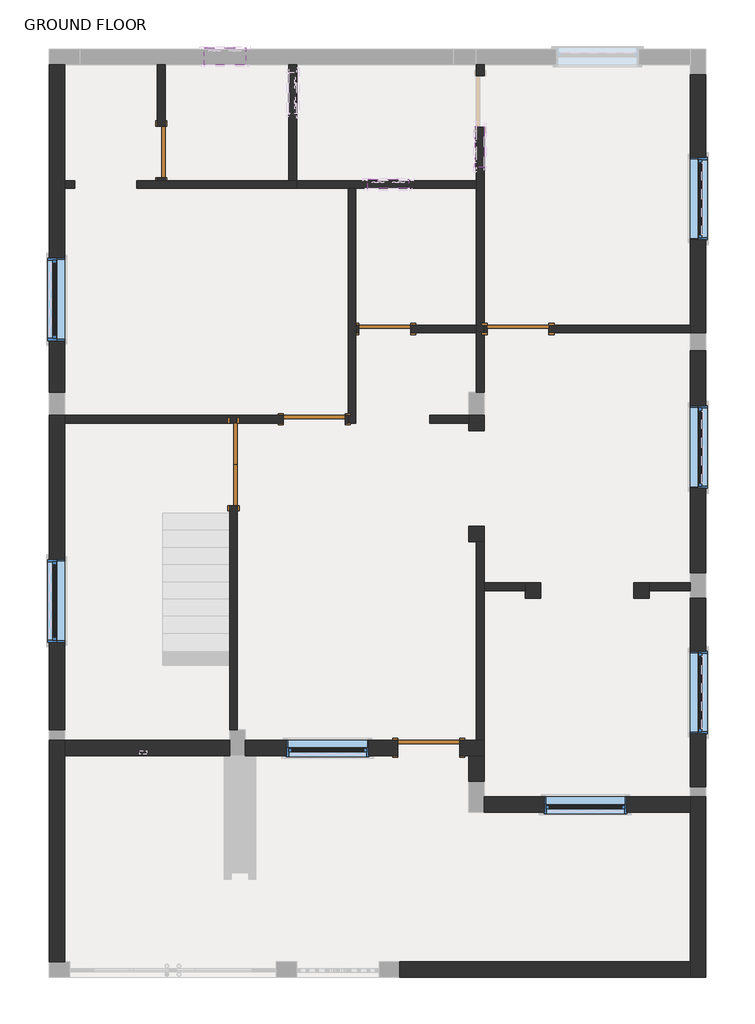
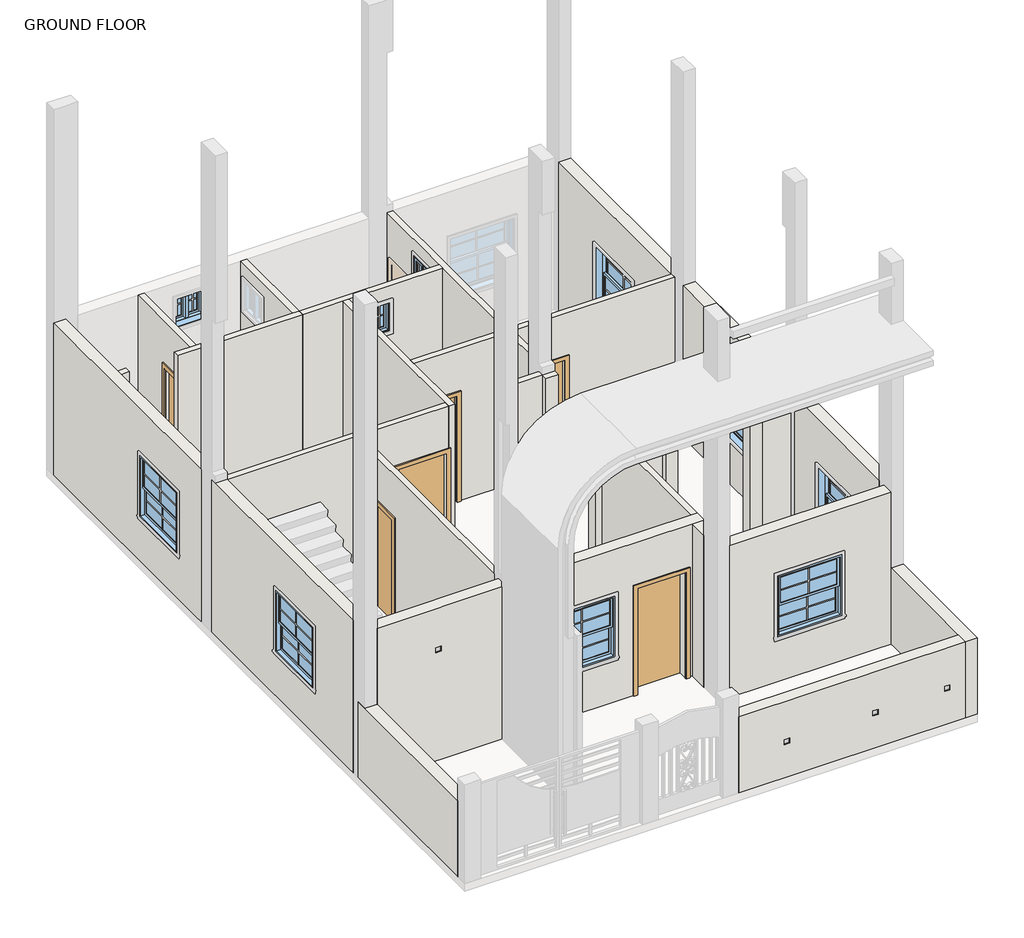
# One storey, part 1 of 3: 31 walls, 10 windows, 6 doors.
"""IFC4 building model written with IfcOpenShell, lengths in millimetres."""

from ifc_helpers import new_model, si_unit, frame, origin, origin_with_axes, place, context, project, spatial, polyline, outline, extrude, faceted_brep, transform, mapped, element, save
from components import door_double_flush_panel_4_x7_eb8a45e1, door_78caadf7, door_214872d5, single_flush_3_x7_0ca8825f, single_flush_3_x7_e5f9f3c4, single_flush_3_x7_305aa2a5, window_casement_double_2_x2_e4709907, window_casement_double_2_x2_3fc3773f, window_double_hung_4_x4_ec8efb0e

model = new_model("IFC4")

# Units and contexts
model_context = context("Model", 3, world=origin())
ifc_project = project(units=[si_unit("LENGTHUNIT", "METRE", prefix="MILLI")], contexts=[model_context])

# Site, building, storey
site = spatial("IfcSite", under=ifc_project)
building = spatial("IfcBuilding", under=site)
storey = spatial("IfcBuildingStorey", under=building, Name="GROUND FLOOR", Elevation=0.0)

# Doors
placement = place(None, origin())
door_double_flush_panel_4_x7_shape = door_double_flush_panel_4_x7_eb8a45e1(model_context)
element("IfcDoor", 1, ObjectType="Door-Double-Flush_Panel : 4'X7'", at=placement, inside=storey, context=model_context, shape_type="MappedRepresentation", body=[
    mapped(door_double_flush_panel_4_x7_shape, transform((-10167.2709734, 2753.6170657, 0.0), x_axis=(0.0, -1.0, 0.0), y_axis=(1.0, 0.0, 0.0), z_axis=(0.0, 0.0, 1.0))),
])
door_shape = door_78caadf7(model_context)
element("IfcDoor", 2, ObjectType="Single-Flush : 2'6\"", at=placement, inside=storey, context=model_context, shape_type="MappedRepresentation", body=[
    mapped(door_shape, transform((-7932.0709734, 4753.8670657, 0.0), x_axis=(-1.0, 0.0, 0.0), y_axis=(0.0, -1.0, 0.0), z_axis=(0.0, 0.0, 1.0))),
])
door_2_shape = door_214872d5(model_context)
element("IfcDoor", 3, ObjectType="Single-Flush : 2'6\"", at=placement, inside=storey, context=model_context, shape_type="MappedRepresentation", body=[
    mapped(door_2_shape, transform((-11234.0709734, 7370.0670657, 0.0), x_axis=(0.0, -1.0, 0.0), y_axis=(1.0, 0.0, 0.0), z_axis=(0.0, 0.0, 1.0))),
])
single_flush_3_x7_shape = single_flush_3_x7_0ca8825f(model_context)
element("IfcDoor", 4, ObjectType="Single-Flush : 3'X7'", at=placement, inside=storey, context=model_context, shape_type="MappedRepresentation", body=[
    mapped(single_flush_3_x7_shape, transform((-7284.3709734, -1437.3829343, 0.0), x_axis=(1.0, 0.0, 0.0), y_axis=(0.0, 1.0, 0.0), z_axis=(0.0, 0.0, 1.0))),
])
single_flush_3_x7_2_shape = single_flush_3_x7_e5f9f3c4(model_context)
element("IfcDoor", 5, ObjectType="Single-Flush : 3'X7'", at=placement, inside=storey, context=model_context, shape_type="MappedRepresentation", body=[
    mapped(single_flush_3_x7_2_shape, transform((-8973.4709734, 3420.3670657, 0.0), x_axis=(1.0, 0.0, 0.0), y_axis=(0.0, 1.0, 0.0), z_axis=(0.0, 0.0, 1.0))),
])
single_flush_3_x7_3_shape = single_flush_3_x7_305aa2a5(model_context)
element("IfcDoor", 6, ObjectType="Single-Flush : 3'X7'", at=placement, inside=storey, context=model_context, shape_type="MappedRepresentation", body=[
    mapped(single_flush_3_x7_3_shape, transform((-5963.5709734, 4753.8670657, 0.0), x_axis=(-1.0, 0.0, 0.0), y_axis=(0.0, -1.0, 0.0), z_axis=(0.0, 0.0, 1.0))),
])

# Walls
element("IfcWall", 7, ObjectType="4.5\"", at=placement, inside=storey, context=model_context, shape_type="SweptSolid", body=[
    extrude(outline(polyline([(-12510.4209734, 6830.3170657), (-12662.8209734, 6830.3170657), (-12662.8209734, 6944.6170657), (-12510.4209734, 6944.6170657), (-12510.4209734, 6830.3170657)])), origin_with_axes(), (0.0, 0.0, 1.0), 3048.0),
])
element("IfcWall", 8, ObjectType="4.5\"", at=placement, inside=storey, context=model_context, shape_type="Brep", body=[
    faceted_brep([(-11596.0209734, 6830.3170657, 0.0), (-9233.8209734, 6830.3170657, 0.0), (-9233.8209734, 6830.3170657, 3048.0), (-11596.0209734, 6830.3170657, 3048.0), (-11596.0209734, 6944.6170657, 0.0), (-11596.0209734, 6944.6170657, 3048.0), (-11291.2209734, 6944.6170657, 3048.0), (-11176.9209734, 6944.6170657, 3048.0), (-9348.1209734, 6944.6170657, 3048.0), (-9233.8209734, 6944.6170657, 3048.0), (-9233.8209734, 6944.6170657, 0.0), (-9348.1209734, 6944.6170657, 0.0), (-11176.9209734, 6944.6170657, 0.0), (-11291.2209734, 6944.6170657, 0.0)], [[[0, 1, 2, 3]], [[4, 5, 6, 7, 8, 9, 10, 11, 12, 13]], [[1, 0, 4, 13, 12, 11, 10]], [[3, 2, 9, 8, 7, 6, 5]], [[0, 3, 5, 4]], [[2, 1, 10, 9]]]),
])
element("IfcWall", 9, ObjectType="4.5\"", at=placement, inside=storey, context=model_context, shape_type="SweptSolid", body=[
    extrude(outline(polyline([(6944.6170657, 0.0), (6944.6170657, 3048.0), (8659.1170657, 3048.0), (8659.1170657, 0.0), (6944.6170657, 0.0)]), holes=[polyline([(7935.2170657, 2743.2), (7935.2170657, 2133.6), (8544.8170657, 2133.6), (8544.8170657, 2743.2), (7935.2170657, 2743.2)])]), frame((-9348.1209734, 0.0, 0.0), z_axis=(1.0, 0.0, 0.0), x_axis=(0.0, 1.0, 0.0)), (0.0, 0.0, 1.0), 114.3),
])
element("IfcWall", 10, ObjectType="4.5\"", at=placement, inside=storey, context=model_context, shape_type="SweptSolid", body=[
    extrude(outline(polyline([(6989.0670657, 2133.6), (6989.0670657, 0.0), (6944.6170657, 0.0), (6944.6170657, 3048.0), (8659.1170657, 3048.0), (8659.1170657, 0.0), (7751.0670657, 0.0), (7751.0670657, 2133.6), (6989.0670657, 2133.6)])), frame((-11291.2209734, 0.0, 0.0), z_axis=(1.0, 0.0, 0.0), x_axis=(0.0, 1.0, 0.0)), (0.0, 0.0, 1.0), 114.3),
])
element("IfcWall", 11, ObjectType="4.5\"", at=placement, inside=storey, context=model_context, shape_type="Brep", body=[
    faceted_brep([(-6579.5209734, 6944.6170657, 0.0), (-9233.8209734, 6944.6170657, 0.0), (-9233.8209734, 6944.6170657, 3048.0), (-6579.5209734, 6944.6170657, 3048.0), (-7576.4709734, 6944.6170657, 2743.2), (-8186.0709734, 6944.6170657, 2743.2), (-8186.0709734, 6944.6170657, 2133.6), (-7576.4709734, 6944.6170657, 2133.6), (-6579.5209734, 6830.3170657, 0.0), (-6579.5209734, 6830.3170657, 3048.0), (-8357.5209734, 6830.3170657, 3048.0), (-8471.8209734, 6830.3170657, 3048.0), (-9233.8209734, 6830.3170657, 3048.0), (-9233.8209734, 6830.3170657, 0.0), (-8471.8209734, 6830.3170657, 0.0), (-8357.5209734, 6830.3170657, 0.0), (-7576.4709734, 6830.3170657, 2743.2), (-7576.4709734, 6830.3170657, 2133.6), (-8186.0709734, 6830.3170657, 2133.6), (-8186.0709734, 6830.3170657, 2743.2)], [[[0, 1, 2, 3], [4, 5, 6, 7]], [[8, 9, 10, 11, 12, 13, 14, 15], [16, 17, 18, 19]], [[1, 0, 8, 15, 14, 13]], [[3, 2, 12, 11, 10, 9]], [[2, 1, 13, 12]], [[0, 3, 9, 8]], [[17, 16, 4, 7]], [[18, 17, 7, 6]], [[19, 18, 6, 5]], [[16, 19, 5, 4]]]),
])
element("IfcWall", 12, ObjectType="4.5\"", at=placement, inside=storey, context=model_context, shape_type="Brep", body=[
    faceted_brep([(-6579.5209734, 3820.4170657, 0.0), (-6579.5209734, 3820.4170657, 3048.0), (-6579.5209734, 4696.7170657, 3048.0), (-6579.5209734, 4811.0170657, 3048.0), (-6579.5209734, 6830.3170657, 3048.0), (-6579.5209734, 6944.6170657, 3048.0), (-6579.5209734, 8659.1170657, 3048.0), (-6579.5209734, 8659.1170657, 0.0), (-6579.5209734, 8494.0170657, 0.0), (-6579.5209734, 8494.0170657, 2133.6), (-6579.5209734, 7751.0670657, 2133.6), (-6579.5209734, 7751.0670657, 2743.2), (-6579.5209734, 7141.4670657, 2743.2), (-6579.5209734, 7141.4670657, 2133.6), (-6579.5209734, 7732.0170657, 2133.6), (-6579.5209734, 7732.0170657, 0.0), (-6579.5209734, 6944.6170657, 0.0), (-6579.5209734, 6830.3170657, 0.0), (-6579.5209734, 4811.0170657, 0.0), (-6579.5209734, 4696.7170657, 0.0), (-6465.2209734, 3820.4170657, 3048.0), (-6465.2209734, 3820.4170657, 0.0), (-6465.2209734, 4696.7170657, 0.0), (-6465.2209734, 4811.0170657, 0.0), (-6465.2209734, 7732.0170657, 0.0), (-6465.2209734, 7732.0170657, 2133.6), (-6465.2209734, 7141.4670657, 2133.6), (-6465.2209734, 7141.4670657, 2743.2), (-6465.2209734, 7751.0670657, 2743.2), (-6465.2209734, 7751.0670657, 2133.6), (-6465.2209734, 8494.0170657, 2133.6), (-6465.2209734, 8494.0170657, 0.0), (-6465.2209734, 8659.1170657, 0.0), (-6465.2209734, 8659.1170657, 3048.0), (-6465.2209734, 4811.0170657, 3048.0), (-6465.2209734, 4696.7170657, 3048.0)], [[[0, 1, 2, 3, 4, 5, 6, 7, 8, 9, 10, 11, 12, 13, 14, 15, 16, 17, 18, 19]], [[20, 21, 22, 23, 24, 25, 26, 27, 28, 29, 30, 31, 32, 33, 34, 35]], [[7, 32, 31, 8]], [[21, 0, 19, 18, 17, 16, 15, 24, 23, 22]], [[1, 0, 21, 20]], [[6, 5, 4, 3, 2, 1, 20, 35, 34, 33]], [[7, 6, 33, 32]], [[9, 8, 31, 30]], [[9, 30, 29, 10]], [[15, 14, 25, 24]], [[28, 11, 10, 29]], [[13, 26, 25, 14]], [[26, 13, 12, 27]], [[11, 28, 27, 12]]]),
])
element("IfcWall", 13, ObjectType="4.5\"", at=placement, inside=storey, context=model_context, shape_type="Brep", body=[
    faceted_brep([(-8471.8209734, 6830.3170657, 0.0), (-8471.8209734, 3477.5170657, 0.0), (-8471.8209734, 3363.2170657, 0.0), (-8471.8209734, 3363.2170657, 3048.0), (-8471.8209734, 3477.5170657, 3048.0), (-8471.8209734, 6830.3170657, 3048.0), (-8357.5209734, 6830.3170657, 0.0), (-8357.5209734, 6830.3170657, 3048.0), (-8357.5209734, 4811.0170657, 3048.0), (-8357.5209734, 4696.7170657, 3048.0), (-8357.5209734, 3363.2170657, 3048.0), (-8357.5209734, 3363.2170657, 0.0), (-8357.5209734, 4696.7170657, 0.0), (-8357.5209734, 4811.0170657, 0.0)], [[[0, 1, 2, 3, 4, 5]], [[6, 7, 8, 9, 10, 11, 12, 13]], [[2, 1, 0, 6, 13, 12, 11]], [[5, 4, 3, 10, 9, 8, 7]], [[0, 5, 7, 6]], [[3, 2, 11, 10]]]),
])
element("IfcWall", 14, ObjectType="4.5\"", at=placement, inside=storey, context=model_context, shape_type="SweptSolid", body=[
    extrude(outline(polyline([(-7265.3209734, 3477.5170657), (-6693.8209734, 3477.5170657), (-6693.8209734, 3363.2170657), (-7265.3209734, 3363.2170657), (-7265.3209734, 3477.5170657)])), origin_with_axes(), (0.0, 0.0, 1.0), 3048.0),
])
element("IfcWall", 15, ObjectType="4.5\"", at=placement, inside=storey, context=model_context, shape_type="SweptSolid", body=[
    extrude(outline(polyline([(0.0, -8357.5209734), (0.0, -8313.0709734), (2133.6, -8313.0709734), (2133.6, -7551.0709734), (0.0, -7551.0709734), (0.0, -6579.5209734), (3048.0, -6579.5209734), (3048.0, -8357.5209734), (0.0, -8357.5209734)])), frame((0.0, 4696.7170657, 0.0), z_axis=(0.0, 1.0, 0.0), x_axis=(0.0, 0.0, 1.0)), (0.0, 0.0, 1.0), 114.3),
])
element("IfcWall", 16, ObjectType="4.5\"", at=placement, inside=storey, context=model_context, shape_type="SweptSolid", body=[
    extrude(outline(polyline([(0.0, -6465.2209734), (0.0, -6420.7709734), (2133.6, -6420.7709734), (2133.6, -5506.3709734), (0.0, -5506.3709734), (0.0, -3417.2209734), (3048.0, -3417.2209734), (3048.0, -6465.2209734), (0.0, -6465.2209734)])), frame((0.0, 4696.7170657, 0.0), z_axis=(0.0, 1.0, 0.0), x_axis=(0.0, 0.0, 1.0)), (0.0, 0.0, 1.0), 114.3),
])
element("IfcWall", 17, ObjectType="4.5\"", at=placement, inside=storey, context=model_context, shape_type="Brep", body=[
    faceted_brep([(-8471.8209734, 3477.5170657, 0.0), (-8516.2709734, 3477.5170657, 0.0), (-8516.2709734, 3477.5170657, 2133.6), (-9430.6709734, 3477.5170657, 2133.6), (-9430.6709734, 3477.5170657, 0.0), (-12662.8209734, 3477.5170657, 0.0), (-12662.8209734, 3477.5170657, 3048.0), (-8471.8209734, 3477.5170657, 3048.0), (-8516.2709734, 3363.2170657, 2133.6), (-8516.2709734, 3363.2170657, 0.0), (-8471.8209734, 3363.2170657, 0.0), (-8471.8209734, 3363.2170657, 3048.0), (-10110.1209734, 3363.2170657, 3048.0), (-10224.4209734, 3363.2170657, 3048.0), (-12662.8209734, 3363.2170657, 3048.0), (-12662.8209734, 3363.2170657, 0.0), (-9430.6709734, 3363.2170657, 0.0), (-9430.6709734, 3363.2170657, 2133.6)], [[[0, 1, 2, 3, 4, 5, 6, 7]], [[8, 9, 10, 11, 12, 13, 14, 15, 16, 17]], [[16, 15, 5, 4]], [[10, 9, 1, 0]], [[7, 6, 14, 13, 12, 11]], [[6, 5, 15, 14]], [[0, 7, 11, 10]], [[2, 1, 9, 8]], [[3, 2, 8, 17]], [[4, 3, 17, 16]]]),
])
element("IfcWall", 18, ObjectType="4.5\"", at=placement, inside=storey, context=model_context, shape_type="SweptSolid", body=[
    extrude(outline(polyline([(-1170.6829343, 3048.0), (3363.2170657, 3048.0), (3363.2170657, 2133.6), (2144.0170657, 2133.6), (2144.0170657, 0.0), (-1170.6829343, 0.0), (-1170.6829343, 3048.0)])), frame((-10224.4209734, 0.0, 0.0), z_axis=(1.0, 0.0, 0.0), x_axis=(0.0, 1.0, 0.0)), (0.0, 0.0, 1.0), 114.3),
])
element("IfcWall", 19, ObjectType="4.5\"", at=placement, inside=storey, context=model_context, shape_type="SweptSolid", body=[
    extrude(outline(polyline([(-4026.8209734, 1001.0170657), (-3417.2209734, 1001.0170657), (-3417.2209734, 886.7170657), (-4026.8209734, 886.7170657), (-4026.8209734, 1001.0170657)])), origin_with_axes(), (0.0, 0.0, 1.0), 3048.0),
])
element("IfcWall", 20, ObjectType="4.5\"", at=placement, inside=storey, context=model_context, shape_type="Brep", body=[
    faceted_brep([(-6579.5209734, 1610.6170657, 0.0), (-6579.5209734, -1323.0829343, 0.0), (-6579.5209734, -1323.0829343, 3048.0), (-6579.5209734, 1610.6170657, 3048.0), (-6465.2209734, 1610.6170657, 0.0), (-6465.2209734, 1610.6170657, 3048.0), (-6465.2209734, 1001.0170657, 3048.0), (-6465.2209734, 886.7170657, 3048.0), (-6465.2209734, -1323.0829343, 3048.0), (-6465.2209734, -1323.0829343, 0.0), (-6465.2209734, 886.7170657, 0.0), (-6465.2209734, 1001.0170657, 0.0)], [[[0, 1, 2, 3]], [[4, 5, 6, 7, 8, 9, 10, 11]], [[1, 0, 4, 11, 10, 9]], [[3, 2, 8, 7, 6, 5]], [[0, 3, 5, 4]], [[2, 1, 9, 8]]]),
])
element("IfcWall", 21, ObjectType="4.5\"", at=placement, inside=storey, context=model_context, shape_type="SweptSolid", body=[
    extrude(outline(polyline([(-5855.6209734, 886.7170657), (-6465.2209734, 886.7170657), (-6465.2209734, 1001.0170657), (-5855.6209734, 1001.0170657), (-5855.6209734, 886.7170657)])), origin_with_axes(), (0.0, 0.0, 1.0), 3048.0),
])
element("IfcWall", 22, ObjectType="9\"", at=placement, inside=storey, context=model_context, shape_type="Brep", body=[
    faceted_brep([(-12891.4209734, 8659.1170657, 0.0), (-12891.4209734, 3820.4170657, 0.0), (-12891.4209734, 3820.4170657, 3048.0), (-12891.4209734, 8659.1170657, 3048.0), (-12891.4209734, 4582.4170657, 2133.6), (-12891.4209734, 4582.4170657, 914.4), (-12891.4209734, 5801.6170657, 914.4), (-12891.4209734, 5801.6170657, 2133.6), (-12662.8209734, 8659.1170657, 0.0), (-12662.8209734, 8659.1170657, 3048.0), (-12662.8209734, 6944.6170657, 3048.0), (-12662.8209734, 6830.3170657, 3048.0), (-12662.8209734, 3820.4170657, 3048.0), (-12662.8209734, 3820.4170657, 0.0), (-12662.8209734, 6830.3170657, 0.0), (-12662.8209734, 6944.6170657, 0.0), (-12662.8209734, 4582.4170657, 2133.6), (-12662.8209734, 5801.6170657, 2133.6), (-12662.8209734, 5801.6170657, 914.4), (-12662.8209734, 4582.4170657, 914.4)], [[[0, 1, 2, 3], [4, 5, 6, 7]], [[8, 9, 10, 11, 12, 13, 14, 15], [16, 17, 18, 19]], [[1, 0, 8, 15, 14, 13]], [[2, 1, 13, 12]], [[3, 2, 12, 11, 10, 9]], [[0, 3, 9, 8]], [[5, 4, 16, 19]], [[6, 5, 19, 18]], [[7, 6, 18, 17]], [[4, 7, 17, 16]]]),
])
element("IfcWall", 23, ObjectType="9\"", at=placement, inside=storey, context=model_context, shape_type="Brep", body=[
    faceted_brep([(-12891.4209734, 3477.5170657, 0.0), (-12891.4209734, -1170.6829343, 0.0), (-12891.4209734, -1170.6829343, 3048.0), (-12891.4209734, 3363.2170657, 3048.0), (-12891.4209734, 3477.5170657, 3048.0), (-12891.4209734, 124.7170657, 2133.6), (-12891.4209734, 124.7170657, 914.4), (-12891.4209734, 1343.9170657, 914.4), (-12891.4209734, 1343.9170657, 2133.6), (-12662.8209734, 3477.5170657, 0.0), (-12662.8209734, 3477.5170657, 3048.0), (-12662.8209734, 3363.2170657, 3048.0), (-12662.8209734, -1170.6829343, 3048.0), (-12662.8209734, -1170.6829343, 0.0), (-12662.8209734, 3363.2170657, 0.0), (-12662.8209734, 124.7170657, 2133.6), (-12662.8209734, 1343.9170657, 2133.6), (-12662.8209734, 1343.9170657, 914.4), (-12662.8209734, 124.7170657, 914.4)], [[[0, 1, 2, 3, 4], [5, 6, 7, 8]], [[9, 10, 11, 12, 13, 14], [15, 16, 17, 18]], [[1, 0, 9, 14, 13]], [[2, 1, 13, 12]], [[4, 3, 2, 12, 11, 10]], [[0, 4, 10, 9]], [[6, 5, 15, 18]], [[7, 6, 18, 17]], [[8, 7, 17, 16]], [[5, 8, 16, 15]]]),
])
element("IfcWall", 24, ObjectType="9\"", at=placement, inside=storey, context=model_context, shape_type="Brep", body=[
    faceted_brep([(-12891.4209734, -1323.0829343, 0.0), (-12891.4209734, -4599.6829343, 0.0), (-12891.4209734, -4599.6829343, 1524.0), (-12891.4209734, -1551.6829343, 1524.0), (-12891.4209734, -1323.0829343, 1524.0), (-12662.8209734, -1323.0829343, 0.0), (-12662.8209734, -1323.0829343, 1524.0), (-12662.8209734, -1551.6829343, 1524.0), (-12662.8209734, -4599.6829343, 1524.0), (-12662.8209734, -4599.6829343, 0.0), (-12662.8209734, -1551.6829343, 0.0)], [[[0, 1, 2, 3, 4]], [[5, 6, 7, 8, 9, 10]], [[1, 0, 5, 10, 9]], [[2, 1, 9, 8]], [[4, 3, 2, 8, 7, 6]], [[0, 4, 6, 5]]]),
])
element("IfcWall", 25, ObjectType="9\"", at=placement, inside=storey, context=model_context, shape_type="Brep", body=[
    faceted_brep([(-3417.2209734, 8506.7170657, 0.0), (-3417.2209734, 4811.0170657, 0.0), (-3417.2209734, 4696.7170657, 0.0), (-3417.2209734, 4696.7170657, 3048.0), (-3417.2209734, 4811.0170657, 3048.0), (-3417.2209734, 8506.7170657, 3048.0), (-3417.2209734, 7287.5170657, 2133.6), (-3417.2209734, 6068.3170657, 2133.6), (-3417.2209734, 6068.3170657, 914.4), (-3417.2209734, 7287.5170657, 914.4), (-3188.6209734, 8506.7170657, 0.0), (-3188.6209734, 8506.7170657, 3048.0), (-3188.6209734, 4811.0170657, 3048.0), (-3188.6209734, 4696.7170657, 3048.0), (-3188.6209734, 4696.7170657, 0.0), (-3188.6209734, 7287.5170657, 2133.6), (-3188.6209734, 7287.5170657, 914.4), (-3188.6209734, 6068.3170657, 914.4), (-3188.6209734, 6068.3170657, 2133.6)], [[[0, 1, 2, 3, 4, 5], [6, 7, 8, 9]], [[10, 11, 12, 13, 14], [15, 16, 17, 18]], [[2, 1, 0, 10, 14]], [[5, 4, 3, 13, 12, 11]], [[0, 5, 11, 10]], [[3, 2, 14, 13]], [[16, 15, 6, 9]], [[17, 16, 9, 8]], [[18, 17, 8, 7]], [[15, 18, 7, 6]]]),
])
element("IfcWall", 26, ObjectType="9\"", at=placement, inside=storey, context=model_context, shape_type="SweptSolid", body=[
    extrude(outline(polyline([(4430.0170657, 0.0), (1153.4170657, 0.0), (1153.4170657, 3048.0), (4430.0170657, 3048.0), (4430.0170657, 0.0)]), holes=[polyline([(3617.2170657, 2133.6), (2398.0170657, 2133.6), (2398.0170657, 914.4), (3617.2170657, 914.4), (3617.2170657, 2133.6)])]), frame((-3417.2209734, 0.0, 0.0), z_axis=(1.0, 0.0, 0.0), x_axis=(0.0, 1.0, 0.0)), (0.0, 0.0, 1.0), 228.6),
])
element("IfcWall", 27, ObjectType="9\"", at=placement, inside=storey, context=model_context, shape_type="SweptSolid", body=[
    extrude(outline(polyline([(772.4170657, 0.0), (-2008.8829343, 0.0), (-2008.8829343, 3048.0), (772.4170657, 3048.0), (772.4170657, 0.0)]), holes=[polyline([(-8.6329343, 2133.6), (-1227.8329343, 2133.6), (-1227.8329343, 914.4), (-8.6329343, 914.4), (-8.6329343, 2133.6)])]), frame((-3417.2209734, 0.0, 0.0), z_axis=(1.0, 0.0, 0.0), x_axis=(0.0, 1.0, 0.0)), (0.0, 0.0, 1.0), 228.6),
])
element("IfcWall", 28, ObjectType="9\"", at=placement, inside=storey, context=model_context, shape_type="Brep", body=[
    faceted_brep([(-3417.2209734, -2161.2829343, 0.0), (-3417.2209734, -2389.8829343, 0.0), (-3417.2209734, -4599.6829343, 0.0), (-3417.2209734, -4828.2829343, 0.0), (-3417.2209734, -4828.2829343, 1524.0), (-3417.2209734, -4599.6829343, 1524.0), (-3417.2209734, -2389.8829343, 1524.0), (-3417.2209734, -2161.2829343, 1524.0), (-3188.6209734, -2161.2829343, 0.0), (-3188.6209734, -2161.2829343, 1524.0), (-3188.6209734, -2389.8829343, 1524.0), (-3188.6209734, -4828.2829343, 1524.0), (-3188.6209734, -4828.2829343, 0.0)], [[[0, 1, 2, 3, 4, 5, 6, 7]], [[8, 9, 10, 11, 12]], [[3, 2, 1, 0, 8, 12]], [[7, 6, 5, 4, 11, 10, 9]], [[4, 3, 12, 11]], [[0, 7, 9, 8]]]),
])
element("IfcWall", 29, ObjectType="9\"", at=placement, inside=storey, context=model_context, shape_type="SweptSolid", body=[
    extrude(outline(polyline([(0.0, -3417.2209734), (1524.0, -3417.2209734), (1524.0, -7709.8209734), (0.0, -7709.8209734), (0.0, -3417.2209734)]), holes=[polyline([(763.994346, -6745.4209734), (663.994346, -6745.4209734), (663.994346, -6845.4209734), (763.994346, -6845.4209734), (763.994346, -6745.4209734)]), polyline([(751.9195264, -5069.0209734), (651.9195264, -5069.0209734), (651.9195264, -5169.0209734), (751.9195264, -5169.0209734), (751.9195264, -5069.0209734)]), polyline([(769.6864335, -3710.1209734), (669.6864335, -3710.1209734), (669.6864335, -3810.1209734), (769.6864335, -3810.1209734), (769.6864335, -3710.1209734)])]), frame((0.0, -4828.2829343, 0.0), z_axis=(0.0, 1.0, 0.0), x_axis=(0.0, 0.0, 1.0)), (0.0, 0.0, 1.0), 228.6),
])
element("IfcWall", 30, ObjectType="9\"", at=placement, inside=storey, context=model_context, shape_type="Brep", body=[
    faceted_brep([(-6827.1709734, -1551.6829343, 2133.6), (-6827.1709734, -1551.6829343, 0.0), (-6693.8209734, -1551.6829343, 0.0), (-6465.2209734, -1551.6829343, 0.0), (-6465.2209734, -1551.6829343, 3048.0), (-6693.8209734, -1551.6829343, 3048.0), (-9995.8209734, -1551.6829343, 3048.0), (-9995.8209734, -1551.6829343, 0.0), (-7741.5709734, -1551.6829343, 0.0), (-7741.5709734, -1551.6829343, 2133.6), (-8167.0209734, -1551.6829343, 2133.6), (-8167.0209734, -1551.6829343, 914.4), (-9386.2209734, -1551.6829343, 914.4), (-9386.2209734, -1551.6829343, 2133.6), (-6465.2209734, -1323.0829343, 0.0), (-6579.5209734, -1323.0829343, 0.0), (-6827.1709734, -1323.0829343, 0.0), (-6827.1709734, -1323.0829343, 2133.6), (-7741.5709734, -1323.0829343, 2133.6), (-7741.5709734, -1323.0829343, 0.0), (-9995.8209734, -1323.0829343, 0.0), (-9995.8209734, -1323.0829343, 3048.0), (-6579.5209734, -1323.0829343, 3048.0), (-6465.2209734, -1323.0829343, 3048.0), (-8167.0209734, -1323.0829343, 2133.6), (-9386.2209734, -1323.0829343, 2133.6), (-9386.2209734, -1323.0829343, 914.4), (-8167.0209734, -1323.0829343, 914.4)], [[[0, 1, 2, 3, 4, 5, 6, 7, 8, 9], [10, 11, 12, 13]], [[14, 15, 16, 17, 18, 19, 20, 21, 22, 23], [24, 25, 26, 27]], [[8, 7, 20, 19]], [[3, 2, 1, 16, 15, 14]], [[6, 5, 4, 23, 22, 21]], [[7, 6, 21, 20]], [[4, 3, 14, 23]], [[17, 16, 1, 0]], [[18, 17, 0, 9]], [[19, 18, 9, 8]], [[11, 10, 24, 27]], [[12, 11, 27, 26]], [[13, 12, 26, 25]], [[10, 13, 25, 24]]]),
])
element("IfcWall", 31, ObjectType="9\"", at=placement, inside=storey, context=model_context, shape_type="Brep", body=[
    faceted_brep([(-6465.2209734, -2389.8829343, 0.0), (-3417.2209734, -2389.8829343, 0.0), (-3417.2209734, -2389.8829343, 1524.0), (-3417.2209734, -2389.8829343, 3048.0), (-6465.2209734, -2389.8829343, 3048.0), (-4357.0209734, -2389.8829343, 2133.6), (-4357.0209734, -2389.8829343, 914.4), (-5576.2209734, -2389.8829343, 914.4), (-5576.2209734, -2389.8829343, 2133.6), (-6465.2209734, -2161.2829343, 0.0), (-6465.2209734, -2161.2829343, 3048.0), (-3417.2209734, -2161.2829343, 3048.0), (-3417.2209734, -2161.2829343, 1524.0), (-3417.2209734, -2161.2829343, 0.0), (-4357.0209734, -2161.2829343, 2133.6), (-5576.2209734, -2161.2829343, 2133.6), (-5576.2209734, -2161.2829343, 914.4), (-4357.0209734, -2161.2829343, 914.4)], [[[0, 1, 2, 3, 4], [5, 6, 7, 8]], [[9, 10, 11, 12, 13], [14, 15, 16, 17]], [[1, 0, 9, 13]], [[4, 3, 11, 10]], [[0, 4, 10, 9]], [[3, 2, 1, 13, 12, 11]], [[6, 5, 14, 17]], [[7, 6, 17, 16]], [[8, 7, 16, 15]], [[5, 8, 15, 14]]]),
])
element("IfcWall", 32, ObjectType="9\"", at=placement, inside=storey, context=model_context, shape_type="Brep", body=[
    faceted_brep([(-6693.8209734, 3477.5170657, 0.0), (-6693.8209734, 3363.2170657, 0.0), (-6693.8209734, 3248.9170657, 0.0), (-6693.8209734, 3248.9170657, 3048.0), (-6693.8209734, 3363.2170657, 3048.0), (-6693.8209734, 3477.5170657, 3048.0), (-6465.2209734, 3477.5170657, 0.0), (-6465.2209734, 3477.5170657, 3048.0), (-6465.2209734, 3363.2170657, 3048.0), (-6465.2209734, 3248.9170657, 3048.0), (-6465.2209734, 3248.9170657, 0.0)], [[[0, 1, 2, 3, 4, 5]], [[6, 7, 8, 9, 10]], [[2, 1, 0, 6, 10]], [[3, 2, 10, 9]], [[5, 4, 3, 9, 8, 7]], [[0, 5, 7, 6]]]),
])
element("IfcWall", 33, ObjectType="9\"", at=placement, inside=storey, context=model_context, shape_type="Brep", body=[
    faceted_brep([(-6693.8209734, 1839.2170657, 0.0), (-6693.8209734, 1610.6170657, 0.0), (-6693.8209734, 1610.6170657, 3048.0), (-6693.8209734, 1839.2170657, 3048.0), (-6465.2209734, 1839.2170657, 0.0), (-6465.2209734, 1839.2170657, 3048.0), (-6465.2209734, 1610.6170657, 3048.0), (-6465.2209734, 1610.6170657, 0.0), (-6579.5209734, 1610.6170657, 0.0), (-6579.5209734, 1610.6170657, 3048.0)], [[[0, 1, 2, 3]], [[4, 5, 6, 7]], [[1, 0, 4, 7, 8]], [[2, 1, 8, 7, 6, 9]], [[3, 2, 9, 6, 5]], [[0, 3, 5, 4]]]),
])
element("IfcWall", 34, ObjectType="9\"", at=placement, inside=storey, context=model_context, shape_type="SweptSolid", body=[
    extrude(outline(polyline([(-6693.8209734, -1932.6829343), (-6693.8209734, -1551.6829343), (-6465.2209734, -1551.6829343), (-6465.2209734, -1932.6829343), (-6693.8209734, -1932.6829343)])), origin_with_axes(), (0.0, 0.0, 1.0), 3048.0),
])
element("IfcWall", 35, ObjectType="9\"", at=placement, inside=storey, context=model_context, shape_type="Brep", body=[
    faceted_brep([(-4255.4209734, 1001.0170657, 0.0), (-4255.4209734, 772.4170657, 0.0), (-4255.4209734, 772.4170657, 3048.0), (-4255.4209734, 1001.0170657, 3048.0), (-4026.8209734, 1001.0170657, 0.0), (-4026.8209734, 1001.0170657, 3048.0), (-4026.8209734, 886.7170657, 3048.0), (-4026.8209734, 772.4170657, 3048.0), (-4026.8209734, 772.4170657, 0.0), (-4026.8209734, 886.7170657, 0.0)], [[[0, 1, 2, 3]], [[4, 5, 6, 7, 8, 9]], [[1, 0, 4, 9, 8]], [[2, 1, 8, 7]], [[3, 2, 7, 6, 5]], [[0, 3, 5, 4]]]),
])
element("IfcWall", 36, ObjectType="9\"", at=placement, inside=storey, context=model_context, shape_type="Brep", body=[
    faceted_brep([(-5627.0209734, 772.4170657, 0.0), (-5627.0209734, 1001.0170657, 0.0), (-5627.0209734, 1001.0170657, 3048.0), (-5627.0209734, 772.4170657, 3048.0), (-5855.6209734, 772.4170657, 0.0), (-5855.6209734, 772.4170657, 3048.0), (-5855.6209734, 886.7170657, 3048.0), (-5855.6209734, 1001.0170657, 3048.0), (-5855.6209734, 1001.0170657, 0.0), (-5855.6209734, 886.7170657, 0.0)], [[[0, 1, 2, 3]], [[4, 5, 6, 7, 8, 9]], [[1, 0, 4, 9, 8]], [[3, 2, 7, 6, 5]], [[0, 3, 5, 4]], [[2, 1, 8, 7]]]),
])
element("IfcWall", 37, ObjectType="9\"", at=placement, inside=storey, context=model_context, shape_type="Brep", body=[
    faceted_brep([(-10224.4209734, -1323.0829343, 0.0), (-12662.8209734, -1323.0829343, 0.0), (-12662.8209734, -1323.0829343, 1524.0), (-12662.8209734, -1323.0829343, 3048.0), (-10224.4209734, -1323.0829343, 3048.0), (-11450.7709734, -1323.0829343, 2267.5734947), (-11550.7709734, -1323.0829343, 2267.5734947), (-11550.7709734, -1323.0829343, 2167.5734947), (-11450.7709734, -1323.0829343, 2167.5734947), (-10224.4209734, -1551.6829343, 0.0), (-10224.4209734, -1551.6829343, 3048.0), (-12662.8209734, -1551.6829343, 3048.0), (-12662.8209734, -1551.6829343, 1524.0), (-12662.8209734, -1551.6829343, 0.0), (-11450.7709734, -1551.6829343, 2267.5734947), (-11450.7709734, -1551.6829343, 2167.5734947), (-11550.7709734, -1551.6829343, 2167.5734947), (-11550.7709734, -1551.6829343, 2267.5734947)], [[[0, 1, 2, 3, 4], [5, 6, 7, 8]], [[9, 10, 11, 12, 13], [14, 15, 16, 17]], [[1, 0, 9, 13]], [[4, 3, 11, 10]], [[0, 4, 10, 9]], [[3, 2, 1, 13, 12, 11]], [[15, 14, 5, 8]], [[16, 15, 8, 7]], [[17, 16, 7, 6]], [[14, 17, 6, 5]]]),
])

# Windows
window_casement_double_2_x2_shape = window_casement_double_2_x2_e4709907(model_context)
element("IfcWindow", 38, ObjectType="Window-Casement-Double : 2'X2'", at=placement, inside=storey, context=model_context, shape_type="MappedRepresentation", body=[
    mapped(window_casement_double_2_x2_shape, transform((-7881.2709734, 6887.4670657, 1219.2), x_axis=(1.0, 0.0, 0.0), y_axis=(0.0, 1.0, 0.0), z_axis=(0.0, 0.0, 1.0))),
])
element("IfcWindow", 39, ObjectType="Window-Casement-Double : 2'X2'", at=placement, inside=storey, context=model_context, shape_type="MappedRepresentation", body=[
    mapped(window_casement_double_2_x2_shape, transform((-6522.3709734, 7446.2670657, 1219.2), x_axis=(0.0, 1.0, 0.0), y_axis=(-1.0, 0.0, 0.0), z_axis=(0.0, 0.0, 1.0))),
])
window_casement_double_2_x2_2_shape = window_casement_double_2_x2_3fc3773f(model_context)
element("IfcWindow", 40, ObjectType="Window-Casement-Double : 2'X2'", at=placement, inside=storey, context=model_context, shape_type="MappedRepresentation", body=[
    mapped(window_casement_double_2_x2_2_shape, transform((-10294.2709734, 8773.4170657, 1219.2), x_axis=(1.0, 0.0, 0.0), y_axis=(0.0, 1.0, 0.0), z_axis=(0.0, 0.0, 1.0))),
])
window_double_hung_4_x4_shape = window_double_hung_4_x4_ec8efb0e(model_context)
element("IfcWindow", 41, ObjectType="Window-Double-Hung : 4'X4'", at=placement, inside=storey, context=model_context, shape_type="MappedRepresentation", body=[
    mapped(window_double_hung_4_x4_shape, transform((-8776.6209734, -1437.3829343, 0.0), x_axis=(-1.0, 0.0, 0.0), y_axis=(0.0, -1.0, 0.0), z_axis=(0.0, 0.0, 1.0))),
])
element("IfcWindow", 42, ObjectType="Window-Double-Hung : 4'X4'", at=placement, inside=storey, context=model_context, shape_type="MappedRepresentation", body=[
    mapped(window_double_hung_4_x4_shape, transform((-12777.1209734, 734.3170657, 0.0), x_axis=(0.0, 1.0, 0.0), y_axis=(-1.0, 0.0, 0.0), z_axis=(0.0, 0.0, 1.0))),
])
element("IfcWindow", 43, ObjectType="Window-Double-Hung : 4'X4'", at=placement, inside=storey, context=model_context, shape_type="MappedRepresentation", body=[
    mapped(window_double_hung_4_x4_shape, transform((-12777.1209734, 5192.0170657, 0.0), x_axis=(0.0, 1.0, 0.0), y_axis=(-1.0, 0.0, 0.0), z_axis=(0.0, 0.0, 1.0))),
])
element("IfcWindow", 44, ObjectType="Window-Double-Hung : 4'X4'", at=placement, inside=storey, context=model_context, shape_type="MappedRepresentation", body=[
    mapped(window_double_hung_4_x4_shape, transform((-3302.9209734, 6677.9170657, 0.0), x_axis=(0.0, -1.0, 0.0), y_axis=(1.0, 0.0, 0.0), z_axis=(0.0, 0.0, 1.0))),
])
element("IfcWindow", 45, ObjectType="Window-Double-Hung : 4'X4'", at=placement, inside=storey, context=model_context, shape_type="MappedRepresentation", body=[
    mapped(window_double_hung_4_x4_shape, transform((-3302.9209734, 3007.6170657, 0.0), x_axis=(0.0, -1.0, 0.0), y_axis=(1.0, 0.0, 0.0), z_axis=(0.0, 0.0, 1.0))),
])
element("IfcWindow", 46, ObjectType="Window-Double-Hung : 4'X4'", at=placement, inside=storey, context=model_context, shape_type="MappedRepresentation", body=[
    mapped(window_double_hung_4_x4_shape, transform((-3302.9209734, -618.2329343, 0.0), x_axis=(0.0, -1.0, 0.0), y_axis=(1.0, 0.0, 0.0), z_axis=(0.0, 0.0, 1.0))),
])
element("IfcWindow", 47, ObjectType="Window-Double-Hung : 4'X4'", at=placement, inside=storey, context=model_context, shape_type="MappedRepresentation", body=[
    mapped(window_double_hung_4_x4_shape, transform((-4966.6209734, -2275.5829343, 0.0), x_axis=(-1.0, 0.0, 0.0), y_axis=(0.0, -1.0, 0.0), z_axis=(0.0, 0.0, 1.0))),
])

save(model, "model.ifc")

# Revit data of these elements
# Type "Door-Double-Flush_Panel : 4'X7'"
#   Type Mark = "11"
#   Construction Type Id = "DOOR"
#   Assembly Code = "C1020"
#   Analytic Construction = "Wooden"
#   Thickness = 0' - 2"
#   Thermal Resistance (R) = 2.5876 (h·ft²·°F)/BTU
#   Swing Angle [instance default] = 90.00°
#   Panel Width = 2' - 0"
#   Heat Transfer Coefficient (U) = 0.3865 BTU/(h·ft²·°F)
#   Height = 7' - 0"
#   Trim Projection Ext = 0' - 1"
#   Trim Projection Int = 0' - 1"
#   Trim Width = 0' - 3"
#   Width = 4' - 0"
#   Define Thermal Properties by = 1
#   Panel Material = Wood - Birch - Solid Stained Light Low Gloss
#   Trim Material = Paint - Sienna
#   Visual Light Transmittance = 0
#   Solar Heat Gain Coefficient = 0
#   Function = (empty or 0)
#   Wall Closure = (empty or 0)
# Type "Single-Flush : 2'6\""
#   Type Mark = "9"
#   Construction Type Id = "MDOOR"
#   Assembly Code = "C1020"
#   Analytic Construction = "Metal"
#   Thickness = 0' - 2"
#   Heat Transfer Coefficient (U) = 0.651978 BTU/(h·ft²·°F)
#   Height = 7' - 0"
#   Trim Projection Ext = 0' - 1"
#   Trim Projection Int = 0' - 1"
#   Trim Width = 0' - 3"
#   Width = 2' - 6"
#   Define Thermal Properties by = 1
#   Door Material = Door - Panel
#   Frame Material = Door - Frame
#   Visual Light Transmittance = 0
#   Solar Heat Gain Coefficient = 0
#   Function = (empty or 0)
#   Wall Closure = (empty or 0)
# Type "Single-Flush : 3'X7'"
#   Type Mark = "8"
#   Construction Type Id = "MDOOR"
#   Assembly Code = "C1020"
#   Analytic Construction = "Metal"
#   Thickness = 0' - 2"
#   Heat Transfer Coefficient (U) = 0.651978 BTU/(h·ft²·°F)
#   Height = 7' - 0"
#   Trim Projection Ext = 0' - 1"
#   Trim Projection Int = 0' - 1"
#   Trim Width = 0' - 3"
#   Width = 3' - 0"
#   Define Thermal Properties by = 1
#   Door Material = Door - Panel
#   Frame Material = Door - Frame
#   Visual Light Transmittance = 0
#   Solar Heat Gain Coefficient = 0
#   Function = (empty or 0)
#   Wall Closure = (empty or 0)
# Type "4.5\""
#   Assembly Code = "B2010"
#   Layers, outside or top first: 0' - 4 1/2" no material (function 1)
# Type "9\""
#   Assembly Code = "B2010"
#   Layers, outside or top first: 0' - 9" no material (function 1)
# Type "Window-Casement-Double : 2'X2'"
#   Type Mark = "20"
#   Fire Rating = "0.5h"
#   Assembly Code = "B2020100"
#   Analytic Construction = "Double glazing - domestic"
#   Frame Extension [instance default] = 0' - 0 1/4"
#   Window Inset [instance default] = 0' - 0"
#   Wall Thickness [instance default] = 0' - 6"
#   Interior Wall Closure [instance default] = 0' - 2 1/4"
#   Half Width = 1' - 0"
#   Visual Light Transmittance = 0.81
#   Thermal Resistance (R) = 1.8146 (h·ft²·°F)/BTU
#   Solar Heat Gain Coefficient = 0.76
#   Rough Width = 2' - 0 1/2"
#   Rough Height = 2' - 0 1/2"
#   Height = 2' - 0"
#   Heat Transfer Coefficient (U) = 0.5511 BTU/(h·ft²·°F)
#   Exterior Wall Closure [instance default] = 0' - 1 1/4"
#   Extension Jamb [instance default] = 0' - 2 1/4"
#   Default Sill Height = 3' - 0"
#   Width = 2' - 0"
#   Muntin Visibility = yes
#   Interior Trim Visibility [instance default] = yes
#   Exterior Trim Visibility [instance default] = yes
#   Extension Jamb Visibility [instance default] = yes
#   Interior Trim Material = Wood - Stained
#   Muntin Pattern = Muntin Pattern_2x2 : Muntin Pattern_2x2
#   Interior Trim = Trim-Window-Interior-Flat : Picture Frame
#   Interior Frame Material = Wood - Stained
#   Glass Panel Material = Glass
#   Exterior Trim Material = Clad - White
#   Exterior Trim = Trim-Window-Exterior-Flat : with Sill
#   Exterior Frame Material = Clad - White
#   Wall Closure = (empty or 0)
# Type "Window-Double-Hung : 4'X4'"
#   Type Mark = "19"
#   Fire Rating = "0.5h"
#   Construction Type Id = "DG-DR"
#   Assembly Code = "B2020100"
#   Analytic Construction = "Double glazing - domestic"
#   Wall Thickness [instance default] = 0' - 6"
#   Window Inset [instance default] = 0' - 0"
#   Visual Light Transmittance = 0.81
#   Thermal Resistance (R) = 1.8146 (h·ft²·°F)/BTU
#   Solar Heat Gain Coefficient = 0.76
#   Muntin Width = 3' - 6"
#   Muntin Height = 1' - 8 1/8"
#   Interior Wall Closure [instance default] = 0' - 1 1/2"
#   Rough Width = 4' - 0 1/2"
#   Rough Height = 4' - 0 1/2"
#   Frame Extension [instance default] = 0' - 1 1/4"
#   Exterior Wall Closure [instance default] = 0' - 0 1/2"
#   Extension Jamb [instance default] = 0' - 1 1/2"
#   Heat Transfer Coefficient (U) = 0.5511 BTU/(h·ft²·°F)
#   Height = 4' - 0"
#   Width = 4' - 0"
#   Top Muntin Visibility = yes
#   Indicator Visibility [instance default] = yes
#   Extension Jamb Visibility [instance default] = yes
#   Interior Trim Visibility [instance default] = yes
#   Exterior Trim Visibility [instance default] = yes
#   Define Thermal Properties by = 1
#   Bottom Muntin Visibility = yes
#   Muntin Pattern = Muntin Pattern_2x2 : Muntin Pattern_2x2
#   Interior Trim Material = Wood - Stained
#   Interior Trim = Trim-Window-Interior-Flat : Picture Frame
#   Exterior Trim Material = Clad - White
#   Exterior Trim = Trim-Window-Exterior-Flat : with Sill
#   Glass Panel Material = Glass
#   Exterior Frame Material = Clad - White
#   Interior Frame Material = Wood - Stained
#   Wall Closure = (empty or 0)
# Element 1 (IfcDoor, "Door-Double-Flush_Panel : 4'X7'")
#   Swing Angle = 90.00°
#   Phase Created = New Construction
#   Materials on its faces: "Paint - Sienna", "Wood - Birch - Solid Stained Light Low Gloss"
# Elements 2, 3 (IfcDoor, "Single-Flush : 2'6\"")
#   Phase Created = New Construction
#   Materials on its faces: "Door - Frame", "Door - Panel"
# Elements 4, 5, 6 (IfcDoor, "Single-Flush : 3'X7'")
#   Phase Created = New Construction
#   Materials on its faces: "Door - Frame", "Door - Panel"
# Elements 7, 8, 9, 10, 11, 12, 13, 14, 15, 16, 17, 18, 19, 20, 21 (IfcWall, "4.5\"")
#   Top Offset = -0' - 6"
#   Base Offset = 0' - 0"
#   wall height = 10' - 0"
#   Phase Created = New Construction
#   Base Constraint = GROUND FLOOR
#   Top Constraint = FIRST FLOOR
#   Materials on its faces: "Default Wall"
# Elements 22, 26, 31 (IfcWall, "9\"")
#   Top Offset = -0' - 6"
#   Base Offset = 0' - 0"
#   wall height = 10' - 0"
#   Phase Created = New Construction
#   Base Constraint = GROUND FLOOR
#   Top Constraint = FIRST FLOOR
#   Materials on its faces: "Default Wall", "Paint - Sienna"
# Elements 23, 25, 27, 30 (IfcWall, "9\"")
#   Top Offset = -0' - 6"
#   Base Offset = 0' - 0"
#   wall height = 10' - 0"
#   Phase Created = New Construction
#   Base Constraint = GROUND FLOOR
#   Top Constraint = FIRST FLOOR
#   Materials on its faces: "Default Wall", "Asphalt, Pavement, Light Grey"
# Elements 24, 28, 29 (IfcWall, "9\"")
#   Top Offset = 0' - 0"
#   Base Offset = 0' - 0"
#   Unconnected Height = 5' - 0"
#   wall height = 5' - 0"
#   Phase Created = New Construction
#   Base Constraint = GROUND FLOOR
#   Materials on its faces: "Default Wall", "EIFS, Exterior Insulation"
# Elements 32, 33, 34, 35, 36 (IfcWall, "9\"")
#   Top Offset = -0' - 6"
#   Base Offset = 0' - 0"
#   wall height = 10' - 0"
#   Phase Created = New Construction
#   Base Constraint = GROUND FLOOR
#   Top Constraint = FIRST FLOOR
#   Materials on its faces: "Default Wall"
# Element 37 (IfcWall, "9\"")
#   Top Offset = -0' - 6"
#   Base Offset = 0' - 0"
#   wall height = 10' - 0"
#   Phase Created = New Construction
#   Base Constraint = GROUND FLOOR
#   Top Constraint = FIRST FLOOR
#   Materials on its faces: "Default Wall", "Softwood, Lumber"
# Element 38 (IfcWindow, "Window-Casement-Double : 2'X2'")
#   Mark = "9"
#   Window Inset = 0' - 0"
#   Interior Wall Closure = 0' - 2 1/4"
#   Frame Extension = 0' - 0 1/4"
#   Exterior Wall Closure = 0' - 1 1/4"
#   Interior Trim Visibility = yes
#   Exterior Trim Visibility = yes
#   Phase Created = New Construction
#   Materials on its faces: "Wood - Stained", "Glass", "Clad - White"
# Element 39 (IfcWindow, "Window-Casement-Double : 2'X2'")
#   Mark = "12"
#   Window Inset = 0' - 0"
#   Interior Wall Closure = 0' - 2 1/4"
#   Frame Extension = 0' - 0 1/4"
#   Exterior Wall Closure = 0' - 1 1/4"
#   Interior Trim Visibility = yes
#   Exterior Trim Visibility = yes
#   Phase Created = New Construction
#   Materials on its faces: "Wood - Stained", "Glass", "Clad - White"
# Element 40 (IfcWindow, "Window-Casement-Double : 2'X2'")
#   Mark = "11"
#   Window Inset = 0' - 0"
#   Interior Wall Closure = 0' - 2 1/4"
#   Frame Extension = 0' - 0 1/4"
#   Exterior Wall Closure = 0' - 1 1/4"
#   Interior Trim Visibility = yes
#   Exterior Trim Visibility = yes
#   Phase Created = New Construction
#   Materials on its faces: "Wood - Stained", "Glass", "Clad - White"
# Element 41 (IfcWindow, "Window-Double-Hung : 4'X4'")
#   Mark = "1"
#   Window Inset = 0' - 0"
#   Interior Wall Closure = 0' - 1 1/2"
#   Frame Extension = 0' - 1 1/4"
#   Exterior Wall Closure = 0' - 0 1/2"
#   Interior Trim Visibility = yes
#   Indicator Visibility = yes
#   Exterior Trim Visibility = yes
#   Phase Created = New Construction
#   Materials on its faces: "Wood - Stained", "Glass", "Clad - White"
# Element 42 (IfcWindow, "Window-Double-Hung : 4'X4'")
#   Mark = "2"
#   Window Inset = 0' - 0"
#   Interior Wall Closure = 0' - 1 1/2"
#   Frame Extension = 0' - 1 1/4"
#   Exterior Wall Closure = 0' - 0 1/2"
#   Interior Trim Visibility = yes
#   Indicator Visibility = yes
#   Exterior Trim Visibility = yes
#   Phase Created = New Construction
#   Materials on its faces: "Wood - Stained", "Glass", "Clad - White"
# Element 43 (IfcWindow, "Window-Double-Hung : 4'X4'")
#   Mark = "3"
#   Window Inset = 0' - 0"
#   Interior Wall Closure = 0' - 1 1/2"
#   Frame Extension = 0' - 1 1/4"
#   Exterior Wall Closure = 0' - 0 1/2"
#   Interior Trim Visibility = yes
#   Indicator Visibility = yes
#   Exterior Trim Visibility = yes
#   Phase Created = New Construction
#   Materials on its faces: "Wood - Stained", "Glass", "Clad - White"
# Element 44 (IfcWindow, "Window-Double-Hung : 4'X4'")
#   Mark = "5"
#   Window Inset = 0' - 0"
#   Interior Wall Closure = 0' - 1 1/2"
#   Frame Extension = 0' - 1 1/4"
#   Exterior Wall Closure = 0' - 0 1/2"
#   Interior Trim Visibility = yes
#   Indicator Visibility = yes
#   Exterior Trim Visibility = yes
#   Phase Created = New Construction
#   Materials on its faces: "Wood - Stained", "Glass", "Clad - White"
# Element 45 (IfcWindow, "Window-Double-Hung : 4'X4'")
#   Mark = "6"
#   Window Inset = 0' - 0"
#   Interior Wall Closure = 0' - 1 1/2"
#   Frame Extension = 0' - 1 1/4"
#   Exterior Wall Closure = 0' - 0 1/2"
#   Interior Trim Visibility = yes
#   Indicator Visibility = yes
#   Exterior Trim Visibility = yes
#   Phase Created = New Construction
#   Materials on its faces: "Wood - Stained", "Glass", "Clad - White"
# Element 46 (IfcWindow, "Window-Double-Hung : 4'X4'")
#   Mark = "7"
#   Window Inset = 0' - 0"
#   Interior Wall Closure = 0' - 1 1/2"
#   Frame Extension = 0' - 1 1/4"
#   Exterior Wall Closure = 0' - 0 1/2"
#   Interior Trim Visibility = yes
#   Indicator Visibility = yes
#   Exterior Trim Visibility = yes
#   Phase Created = New Construction
#   Materials on its faces: "Wood - Stained", "Glass", "Clad - White"
# Element 47 (IfcWindow, "Window-Double-Hung : 4'X4'")
#   Mark = "8"
#   Window Inset = 0' - 0"
#   Interior Wall Closure = 0' - 1 1/2"
#   Frame Extension = 0' - 1 1/4"
#   Exterior Wall Closure = 0' - 0 1/2"
#   Interior Trim Visibility = yes
#   Indicator Visibility = yes
#   Exterior Trim Visibility = yes
#   Phase Created = New Construction
#   Materials on its faces: "Wood - Stained", "Glass", "Clad - White"
# Materials
#   "Wood - Birch - Solid Stained Light Low Gloss": class "Wood", colour RGB 210 159 95, transparency 0, Cost = 0
#   "Paint - Sienna": colour RGB 118 70 51, transparency 0, Cost = 0
#   "Door - Panel": class "Wood", colour RGB 210 159 95, transparency 0, Cost = 0
#   "Door - Frame": colour RGB 118 70 51, transparency 0, Cost = 0
#   "Wood - Stained": class "Wood", colour RGB 224 178 126, transparency 0, Cost = 0
#   "Glass": class "Glass", colour RGB 0 128 192, transparency 0.75, Description = "Soda Lime Glass", Cost = 0
#   "Clad - White": class "Wood", colour RGB 242 242 238, transparency 0, Cost = 0
#   "Default Wall": colour RGB 128 128 128, transparency 0, Cost = 0
#   "Asphalt, Pavement, Light Grey": class "Generic", colour RGB 120 120 120, transparency 0, Description = "Asphalt or tarmac paving", Cost = 0
#   "EIFS, Exterior Insulation": class "Generic", colour RGB 127 127 127, transparency 0, Description = "EIFS - Exterior Insulation", Cost = 0
#   "Softwood, Lumber": class "Wood", colour RGB 223 192 134, transparency 0, Description = "Pinus Echinata", Cost = 0
